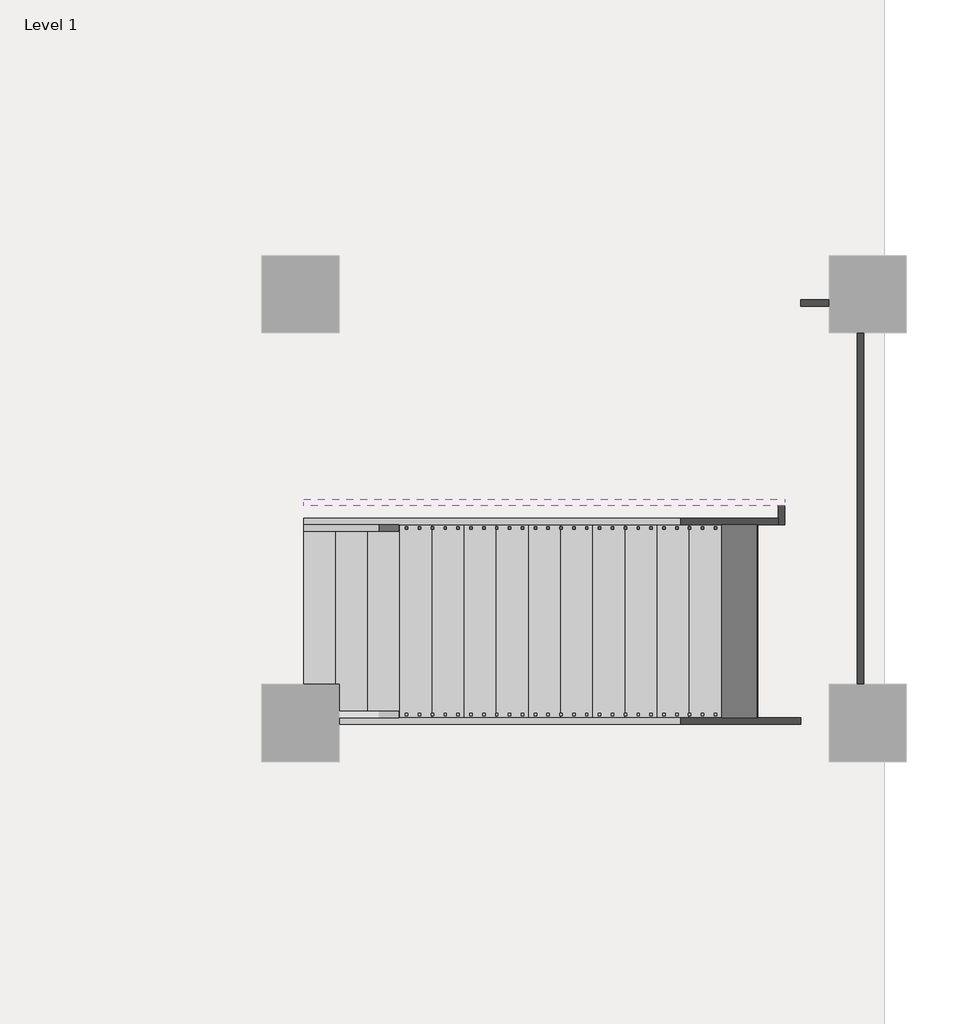
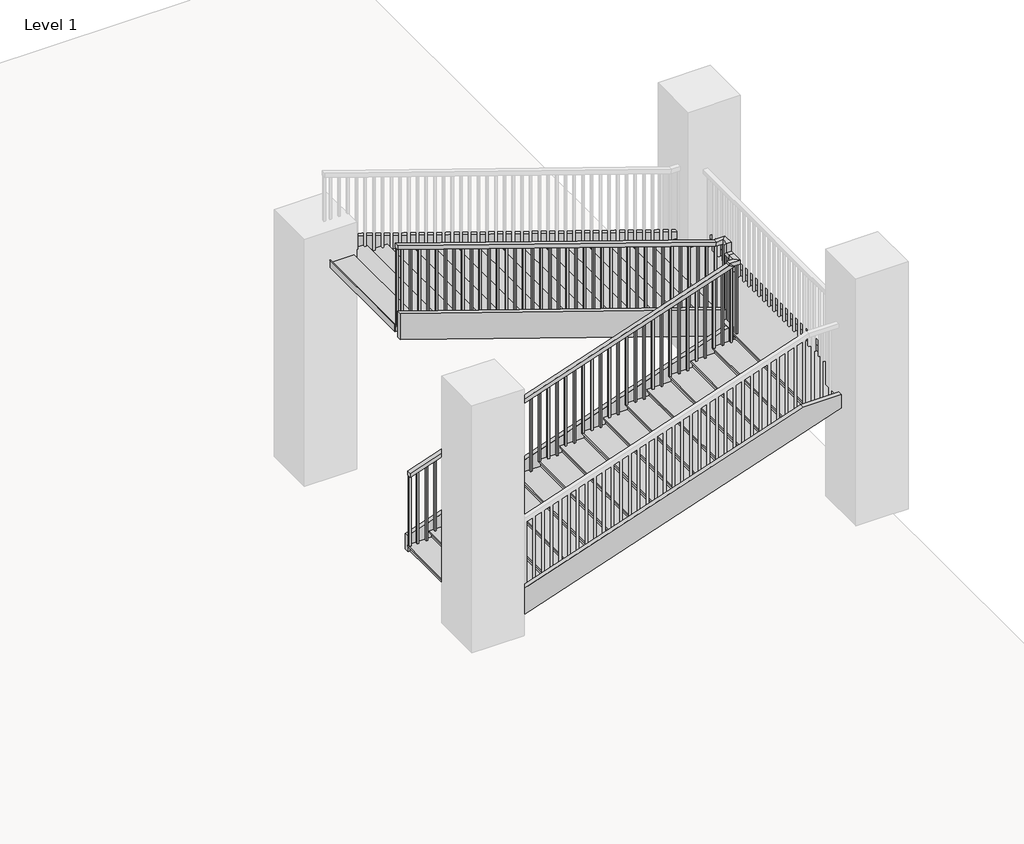
# One storey, part 2 of 2: 6 members, 1 railing, 1 stair flight.
"""IFC4 building model written with IfcOpenShell, lengths in millimetres."""

from ifc_helpers import new_model, si_unit, frame, origin, place, context, project, spatial, polyline, outline, extrude, faceted_brep, transform, mapped, element, save
from components import stair_flight_62363484

model = new_model("IFC4")

# Units and contexts
model_context = context("Model", 3, world=origin())
ifc_project = project(units=[si_unit("LENGTHUNIT", "METRE", prefix="MILLI")], contexts=[model_context])

# Site, building, storey
site = spatial("IfcSite", under=ifc_project)
building = spatial("IfcBuilding", under=site)
storey = spatial("IfcBuildingStorey", under=building, Name="Level 1", Elevation=0.0)

# Members
placement = place(None, origin())
element("IfcMember", 1, ObjectType="Stringer - 2\" Width", at=placement, inside=storey, context=model_context, shape_type="SweptSolid", body=[
    extrude(outline(polyline([(193.7751932, 1449.3932247), (0.0, 1449.3932247), (0.0, 1827.5890963), (1140.094539, 5195.8669505), (1447.8, 5195.8669505), (1447.8, 5154.2649181), (193.7751932, 1449.3932247)])), frame((0.0, -541.2659014, 0.0), z_axis=(0.0, 1.0, 0.0), x_axis=(0.0, 0.0, 1.0)), (0.0, 0.0, 1.0), 50.8),
])
element("IfcMember", 2, ObjectType="Stringer - 2\" Width", at=placement, inside=storey, context=model_context, shape_type="SweptSolid", body=[
    extrude(outline(polyline([(5246.6669505, -541.2659014), (5195.8669505, -541.2659014), (5195.8669505, -388.7910016), (5246.6669505, -388.7910016), (5246.6669505, -541.2659014)])), frame((0.0, 0.0, 1143.0), z_axis=(0.0, 0.0, 1.0), x_axis=(1.0, 0.0, 0.0)), (0.0, 0.0, 1.0), 304.8),
])
element("IfcMember", 3, ObjectType="Stringer - 2\" Width", at=placement, inside=storey, context=model_context, shape_type="SweptSolid", body=[
    extrude(outline(polyline([(1243.0143208, 5246.6669505), (1564.8012358, 5246.6669505), (2850.1022784, 1449.3932247), (2528.3153634, 1449.3932247), (1243.0143208, 5246.6669505)])), frame((0.0, -388.7910016, 0.0), z_axis=(0.0, 1.0, 0.0), x_axis=(0.0, 0.0, 1.0)), (0.0, 0.0, 1.0), 50.8),
])
element("IfcMember", 4, ObjectType="Stringer - 2\" Width", at=placement, inside=storey, context=model_context, shape_type="SweptSolid", body=[
    extrude(outline(polyline([(193.7751932, 1449.3932247), (0.0, 1449.3932247), (0.0, 1827.5890963), (1352.1142723, 5822.2548051), (1447.8, 5822.2548051), (1447.8, 5154.2649181), (193.7751932, 1449.3932247)])), frame((0.0, -2116.0659014, 0.0), z_axis=(0.0, 1.0, 0.0), x_axis=(0.0, 0.0, 1.0)), (0.0, 0.0, 1.0), 50.8),
])
element("IfcMember", 5, ObjectType="Stringer - 2\" Width", at=placement, inside=storey, context=model_context, shape_type="SweptSolid", body=[
    extrude(outline(polyline([(5873.0548051, -2116.0659014), (5822.2548051, -2116.0659014), (5822.2548051, 1185.9340986), (5873.0548051, 1185.9340986), (5873.0548051, -2116.0659014)])), frame((0.0, 0.0, 1143.0), z_axis=(0.0, 0.0, 1.0), x_axis=(1.0, 0.0, 0.0)), (0.0, 0.0, 1.0), 304.8),
])
element("IfcMember", 6, ObjectType="Stringer - 2\" Width", at=placement, inside=storey, context=model_context, shape_type="SweptSolid", body=[
    extrude(outline(polyline([(1143.0, 5873.0548051), (1352.7815025, 5873.0548051), (2850.1022784, 1449.3932247), (2528.3153634, 1449.3932247), (1143.0, 5542.1477288), (1143.0, 5873.0548051)])), frame((0.0, 1185.9340986, 0.0), z_axis=(0.0, 1.0, 0.0), x_axis=(0.0, 0.0, 1.0)), (0.0, 0.0, 1.0), 50.8),
])

# Railing
element("IfcRailing", 7, ObjectType="Handrail - Rectangular", at=placement, inside=storey, context=model_context, shape_type="SolidModel", body=[
    faceted_brep([(1449.3932247, -541.2659014, 1000.125), (1449.3932247, -541.2659014, 946.4913852), (1449.3932247, -592.0659014, 946.4913852), (1449.3932247, -592.0659014, 1000.125), (5170.4669505, -541.2659014, 2260.1963098), (5221.2669505, -541.2659014, 2223.7651551), (5221.2669505, -592.0659014, 2223.7651551), (5170.4669505, -592.0659014, 2260.1963098), (5170.4669505, -541.2659014, 2286.0), (5221.2669505, -541.2659014, 2235.2), (5221.2669505, -592.0659014, 2235.2), (5170.4669505, -592.0659014, 2286.0), (5246.6669505, -541.2659014, 2286.0), (5246.6669505, -541.2659014, 2235.2), (5297.4669505, -592.0659014, 2235.2), (5297.4669505, -592.0659014, 2286.0), (5246.6669505, -465.0659014, 2286.0), (5246.6669505, -465.0659014, 2235.2), (5297.4669505, -465.0659014, 2235.2), (5297.4669505, -465.0659014, 2286.0), (5246.6669505, -414.1910016, 2286.0), (5246.6669505, -363.3910016, 2235.2), (5297.4669505, -363.3910016, 2235.2), (5297.4669505, -414.1910016, 2286.0), (5246.6669505, -414.1910016, 2397.5286902), (5246.6669505, -363.3910016, 2346.7286902), (5297.4669505, -363.3910016, 2346.7286902), (5297.4669505, -414.1910016, 2397.5286902), (5246.6669505, -337.9910016, 2397.5286902), (5246.6669505, -337.9910016, 2346.7286902), (5297.4669505, -287.1910016, 2346.7286902), (5297.4669505, -287.1910016, 2397.5286902), (5170.4669505, -337.9910016, 2397.5286902), (5162.099099, -337.9910016, 2346.7286902), (5162.099099, -287.1910016, 2346.7286902), (5170.4669505, -287.1910016, 2397.5286902), (1449.3932247, -337.9910016, 3657.6), (1449.3932247, -287.1910016, 3657.6), (1449.3932247, -287.1910016, 3603.9663852), (1449.3932247, -337.9910016, 3603.9663852)], [[[0, 1, 2, 3]], [[1, 0, 4, 5]], [[2, 1, 5, 6]], [[3, 2, 6, 7]], [[0, 3, 7, 4]], [[5, 4, 8, 9]], [[6, 5, 9, 10]], [[7, 6, 10, 11]], [[4, 7, 11, 8]], [[9, 8, 12, 13]], [[10, 9, 13, 14]], [[11, 10, 14, 15]], [[8, 11, 15, 12]], [[13, 12, 16, 17]], [[14, 13, 17, 18]], [[15, 14, 18, 19]], [[12, 15, 19, 16]], [[17, 16, 20, 21]], [[18, 17, 21, 22]], [[19, 18, 22, 23]], [[16, 19, 23, 20]], [[21, 20, 24, 25]], [[22, 21, 25, 26]], [[23, 22, 26, 27]], [[20, 23, 27, 24]], [[25, 24, 28, 29]], [[26, 25, 29, 30]], [[27, 26, 30, 31]], [[24, 27, 31, 28]], [[29, 28, 32, 33]], [[30, 29, 33, 34]], [[31, 30, 34, 35]], [[28, 31, 35, 32]], [[36, 37, 38, 39]], [[33, 32, 36, 39]], [[34, 33, 39, 38]], [[35, 34, 38, 37]], [[32, 35, 37, 36]]]),
    extrude(outline(polyline([(3585.6976686, 1503.3419505), (2657.475, 1503.3419505), (2657.475, 1522.3919505), (3579.246746, 1522.3919505), (3585.6976686, 1503.3419505)])), frame((0.0, -322.1160016, 0.0), z_axis=(0.0, 1.0, 0.0), x_axis=(0.0, 0.0, 1.0)), (0.0, 0.0, 1.0), 19.05),
    extrude(outline(polyline([(3551.2927482, 1604.9419505), (2657.475, 1604.9419505), (2657.475, 1623.9919505), (3544.8418257, 1623.9919505), (3551.2927482, 1604.9419505)])), frame((0.0, -322.1160016, 0.0), z_axis=(0.0, 1.0, 0.0), x_axis=(0.0, 0.0, 1.0)), (0.0, 0.0, 1.0), 19.05),
    extrude(outline(polyline([(3516.8878279, 1706.5419505), (2571.75, 1706.5419505), (2571.75, 1725.5919505), (3510.4369054, 1725.5919505), (3516.8878279, 1706.5419505)])), frame((0.0, -322.1160016, 0.0), z_axis=(0.0, 1.0, 0.0), x_axis=(0.0, 0.0, 1.0)), (0.0, 0.0, 1.0), 19.05),
    extrude(outline(polyline([(3482.4829076, 1808.1419505), (2571.75, 1808.1419505), (2571.75, 1827.1919505), (3476.031985, 1827.1919505), (3482.4829076, 1808.1419505)])), frame((0.0, -322.1160016, 0.0), z_axis=(0.0, 1.0, 0.0), x_axis=(0.0, 0.0, 1.0)), (0.0, 0.0, 1.0), 19.05),
    extrude(outline(polyline([(3448.0779873, 1909.7419505), (2571.75, 1909.7419505), (2571.75, 1928.7919505), (3441.6270647, 1928.7919505), (3448.0779873, 1909.7419505)])), frame((0.0, -322.1160016, 0.0), z_axis=(0.0, 1.0, 0.0), x_axis=(0.0, 0.0, 1.0)), (0.0, 0.0, 1.0), 19.05),
    extrude(outline(polyline([(3413.6730669, 2011.3419505), (2486.025, 2011.3419505), (2486.025, 2030.3919505), (3407.2221444, 2030.3919505), (3413.6730669, 2011.3419505)])), frame((0.0, -322.1160016, 0.0), z_axis=(0.0, 1.0, 0.0), x_axis=(0.0, 0.0, 1.0)), (0.0, 0.0, 1.0), 19.05),
    extrude(outline(polyline([(3379.2681466, 2112.9419505), (2486.025, 2112.9419505), (2486.025, 2131.9919505), (3372.817224, 2131.9919505), (3379.2681466, 2112.9419505)])), frame((0.0, -322.1160016, 0.0), z_axis=(0.0, 1.0, 0.0), x_axis=(0.0, 0.0, 1.0)), (0.0, 0.0, 1.0), 19.05),
    extrude(outline(polyline([(3344.8632263, 2214.5419505), (2400.3, 2214.5419505), (2400.3, 2233.5919505), (3338.4123037, 2233.5919505), (3344.8632263, 2214.5419505)])), frame((0.0, -322.1160016, 0.0), z_axis=(0.0, 1.0, 0.0), x_axis=(0.0, 0.0, 1.0)), (0.0, 0.0, 1.0), 19.05),
    extrude(outline(polyline([(3310.4583059, 2316.1419505), (2400.3, 2316.1419505), (2400.3, 2335.1919505), (3304.0073834, 2335.1919505), (3310.4583059, 2316.1419505)])), frame((0.0, -322.1160016, 0.0), z_axis=(0.0, 1.0, 0.0), x_axis=(0.0, 0.0, 1.0)), (0.0, 0.0, 1.0), 19.05),
    extrude(outline(polyline([(3276.0533856, 2417.7419505), (2400.3, 2417.7419505), (2400.3, 2436.7919505), (3269.6024631, 2436.7919505), (3276.0533856, 2417.7419505)])), frame((0.0, -322.1160016, 0.0), z_axis=(0.0, 1.0, 0.0), x_axis=(0.0, 0.0, 1.0)), (0.0, 0.0, 1.0), 19.05),
    extrude(outline(polyline([(3241.6484653, 2519.3419505), (2314.575, 2519.3419505), (2314.575, 2538.3919505), (3235.1975427, 2538.3919505), (3241.6484653, 2519.3419505)])), frame((0.0, -322.1160016, 0.0), z_axis=(0.0, 1.0, 0.0), x_axis=(0.0, 0.0, 1.0)), (0.0, 0.0, 1.0), 19.05),
    extrude(outline(polyline([(3207.243545, 2620.9419505), (2314.575, 2620.9419505), (2314.575, 2639.9919505), (3200.7926224, 2639.9919505), (3207.243545, 2620.9419505)])), frame((0.0, -322.1160016, 0.0), z_axis=(0.0, 1.0, 0.0), x_axis=(0.0, 0.0, 1.0)), (0.0, 0.0, 1.0), 19.05),
    extrude(outline(polyline([(3172.8386246, 2722.5419505), (2228.85, 2722.5419505), (2228.85, 2741.5919505), (3166.3877021, 2741.5919505), (3172.8386246, 2722.5419505)])), frame((0.0, -322.1160016, 0.0), z_axis=(0.0, 1.0, 0.0), x_axis=(0.0, 0.0, 1.0)), (0.0, 0.0, 1.0), 19.05),
    extrude(outline(polyline([(3138.4337043, 2824.1419505), (2228.85, 2824.1419505), (2228.85, 2843.1919505), (3131.9827817, 2843.1919505), (3138.4337043, 2824.1419505)])), frame((0.0, -322.1160016, 0.0), z_axis=(0.0, 1.0, 0.0), x_axis=(0.0, 0.0, 1.0)), (0.0, 0.0, 1.0), 19.05),
    extrude(outline(polyline([(3104.028784, 2925.7419505), (2228.85, 2925.7419505), (2228.85, 2944.7919505), (3097.5778614, 2944.7919505), (3104.028784, 2925.7419505)])), frame((0.0, -322.1160016, 0.0), z_axis=(0.0, 1.0, 0.0), x_axis=(0.0, 0.0, 1.0)), (0.0, 0.0, 1.0), 19.05),
    extrude(outline(polyline([(3069.6238636, 3027.3419505), (2143.125, 3027.3419505), (2143.125, 3046.3919505), (3063.1729411, 3046.3919505), (3069.6238636, 3027.3419505)])), frame((0.0, -322.1160016, 0.0), z_axis=(0.0, 1.0, 0.0), x_axis=(0.0, 0.0, 1.0)), (0.0, 0.0, 1.0), 19.05),
    extrude(outline(polyline([(3035.2189433, 3128.9419505), (2143.125, 3128.9419505), (2143.125, 3147.9919505), (3028.7680208, 3147.9919505), (3035.2189433, 3128.9419505)])), frame((0.0, -322.1160016, 0.0), z_axis=(0.0, 1.0, 0.0), x_axis=(0.0, 0.0, 1.0)), (0.0, 0.0, 1.0), 19.05),
    extrude(outline(polyline([(3000.814023, 3230.5419505), (2057.4, 3230.5419505), (2057.4, 3249.5919505), (2994.3631004, 3249.5919505), (3000.814023, 3230.5419505)])), frame((0.0, -322.1160016, 0.0), z_axis=(0.0, 1.0, 0.0), x_axis=(0.0, 0.0, 1.0)), (0.0, 0.0, 1.0), 19.05),
    extrude(outline(polyline([(2966.4091027, 3332.1419505), (2057.4, 3332.1419505), (2057.4, 3351.1919505), (2959.9581801, 3351.1919505), (2966.4091027, 3332.1419505)])), frame((0.0, -322.1160016, 0.0), z_axis=(0.0, 1.0, 0.0), x_axis=(0.0, 0.0, 1.0)), (0.0, 0.0, 1.0), 19.05),
    extrude(outline(polyline([(2932.0041823, 3433.7419505), (2057.4, 3433.7419505), (2057.4, 3452.7919505), (2925.5532598, 3452.7919505), (2932.0041823, 3433.7419505)])), frame((0.0, -322.1160016, 0.0), z_axis=(0.0, 1.0, 0.0), x_axis=(0.0, 0.0, 1.0)), (0.0, 0.0, 1.0), 19.05),
    extrude(outline(polyline([(2897.599262, 3535.3419505), (1971.675, 3535.3419505), (1971.675, 3554.3919505), (2891.1483394, 3554.3919505), (2897.599262, 3535.3419505)])), frame((0.0, -322.1160016, 0.0), z_axis=(0.0, 1.0, 0.0), x_axis=(0.0, 0.0, 1.0)), (0.0, 0.0, 1.0), 19.05),
    extrude(outline(polyline([(2863.1943417, 3636.9419505), (1971.675, 3636.9419505), (1971.675, 3655.9919505), (2856.7434191, 3655.9919505), (2863.1943417, 3636.9419505)])), frame((0.0, -322.1160016, 0.0), z_axis=(0.0, 1.0, 0.0), x_axis=(0.0, 0.0, 1.0)), (0.0, 0.0, 1.0), 19.05),
    extrude(outline(polyline([(2828.7894213, 3738.5419505), (1885.95, 3738.5419505), (1885.95, 3757.5919505), (2822.3384988, 3757.5919505), (2828.7894213, 3738.5419505)])), frame((0.0, -322.1160016, 0.0), z_axis=(0.0, 1.0, 0.0), x_axis=(0.0, 0.0, 1.0)), (0.0, 0.0, 1.0), 19.05),
    extrude(outline(polyline([(2794.384501, 3840.1419505), (1885.95, 3840.1419505), (1885.95, 3859.1919505), (2787.9335784, 3859.1919505), (2794.384501, 3840.1419505)])), frame((0.0, -322.1160016, 0.0), z_axis=(0.0, 1.0, 0.0), x_axis=(0.0, 0.0, 1.0)), (0.0, 0.0, 1.0), 19.05),
    extrude(outline(polyline([(2759.9795807, 3941.7419505), (1885.95, 3941.7419505), (1885.95, 3960.7919505), (2753.5286581, 3960.7919505), (2759.9795807, 3941.7419505)])), frame((0.0, -322.1160016, 0.0), z_axis=(0.0, 1.0, 0.0), x_axis=(0.0, 0.0, 1.0)), (0.0, 0.0, 1.0), 19.05),
    extrude(outline(polyline([(2725.5746604, 4043.3419505), (1800.225, 4043.3419505), (1800.225, 4062.3919505), (2719.1237378, 4062.3919505), (2725.5746604, 4043.3419505)])), frame((0.0, -322.1160016, 0.0), z_axis=(0.0, 1.0, 0.0), x_axis=(0.0, 0.0, 1.0)), (0.0, 0.0, 1.0), 19.05),
    extrude(outline(polyline([(2691.16974, 4144.9419505), (1800.225, 4144.9419505), (1800.225, 4163.9919505), (2684.7188175, 4163.9919505), (2691.16974, 4144.9419505)])), frame((0.0, -322.1160016, 0.0), z_axis=(0.0, 1.0, 0.0), x_axis=(0.0, 0.0, 1.0)), (0.0, 0.0, 1.0), 19.05),
    extrude(outline(polyline([(2656.7648197, 4246.5419505), (1714.5, 4246.5419505), (1714.5, 4265.5919505), (2650.3138971, 4265.5919505), (2656.7648197, 4246.5419505)])), frame((0.0, -322.1160016, 0.0), z_axis=(0.0, 1.0, 0.0), x_axis=(0.0, 0.0, 1.0)), (0.0, 0.0, 1.0), 19.05),
    extrude(outline(polyline([(2622.3598994, 4348.1419505), (1714.5, 4348.1419505), (1714.5, 4367.1919505), (2615.9089768, 4367.1919505), (2622.3598994, 4348.1419505)])), frame((0.0, -322.1160016, 0.0), z_axis=(0.0, 1.0, 0.0), x_axis=(0.0, 0.0, 1.0)), (0.0, 0.0, 1.0), 19.05),
    extrude(outline(polyline([(2587.954979, 4449.7419505), (1714.5, 4449.7419505), (1714.5, 4468.7919505), (2581.5040565, 4468.7919505), (2587.954979, 4449.7419505)])), frame((0.0, -322.1160016, 0.0), z_axis=(0.0, 1.0, 0.0), x_axis=(0.0, 0.0, 1.0)), (0.0, 0.0, 1.0), 19.05),
    extrude(outline(polyline([(2553.5500587, 4551.3419505), (1628.775, 4551.3419505), (1628.775, 4570.3919505), (2547.0991361, 4570.3919505), (2553.5500587, 4551.3419505)])), frame((0.0, -322.1160016, 0.0), z_axis=(0.0, 1.0, 0.0), x_axis=(0.0, 0.0, 1.0)), (0.0, 0.0, 1.0), 19.05),
    extrude(outline(polyline([(2519.1451384, 4652.9419505), (1628.775, 4652.9419505), (1628.775, 4671.9919505), (2512.6942158, 4671.9919505), (2519.1451384, 4652.9419505)])), frame((0.0, -322.1160016, 0.0), z_axis=(0.0, 1.0, 0.0), x_axis=(0.0, 0.0, 1.0)), (0.0, 0.0, 1.0), 19.05),
    extrude(outline(polyline([(2484.7402181, 4754.5419505), (1543.05, 4754.5419505), (1543.05, 4773.5919505), (2478.2892955, 4773.5919505), (2484.7402181, 4754.5419505)])), frame((0.0, -322.1160016, 0.0), z_axis=(0.0, 1.0, 0.0), x_axis=(0.0, 0.0, 1.0)), (0.0, 0.0, 1.0), 19.05),
    extrude(outline(polyline([(2450.3352977, 4856.1419505), (1543.05, 4856.1419505), (1543.05, 4875.1919505), (2443.8843752, 4875.1919505), (2450.3352977, 4856.1419505)])), frame((0.0, -322.1160016, 0.0), z_axis=(0.0, 1.0, 0.0), x_axis=(0.0, 0.0, 1.0)), (0.0, 0.0, 1.0), 19.05),
    extrude(outline(polyline([(2415.9303774, 4957.7419505), (1543.05, 4957.7419505), (1543.05, 4976.7919505), (2409.4794548, 4976.7919505), (2415.9303774, 4957.7419505)])), frame((0.0, -322.1160016, 0.0), z_axis=(0.0, 1.0, 0.0), x_axis=(0.0, 0.0, 1.0)), (0.0, 0.0, 1.0), 19.05),
    extrude(outline(polyline([(2381.5254571, 5059.3419505), (1457.325, 5059.3419505), (1457.325, 5078.3919505), (2375.0745345, 5078.3919505), (2381.5254571, 5059.3419505)])), frame((0.0, -322.1160016, 0.0), z_axis=(0.0, 1.0, 0.0), x_axis=(0.0, 0.0, 1.0)), (0.0, 0.0, 1.0), 19.05),
    extrude(outline(polyline([(2347.1205367, 5160.9419505), (1457.325, 5160.9419505), (1457.325, 5179.9919505), (2340.6696142, 5179.9919505), (2347.1205367, 5160.9419505)])), frame((0.0, -322.1160016, 0.0), z_axis=(0.0, 1.0, 0.0), x_axis=(0.0, 0.0, 1.0)), (0.0, 0.0, 1.0), 19.05),
    extrude(outline(polyline([(5262.5419505, -372.9909014), (5262.5419505, -353.9409014), (5281.5919505, -353.9409014), (5281.5919505, -372.9909014), (5262.5419505, -372.9909014)])), frame((0.0, 0.0, 1371.6), z_axis=(0.0, 0.0, 1.0), x_axis=(1.0, 0.0, 0.0)), (0.0, 0.0, 1.0), 975.1286902),
    extrude(outline(polyline([(5262.5419505, -474.5909014), (5262.5419505, -455.5409014), (5281.5919505, -455.5409014), (5281.5919505, -474.5909014), (5262.5419505, -474.5909014)])), frame((0.0, 0.0, 1371.6), z_axis=(0.0, 0.0, 1.0), x_axis=(1.0, 0.0, 0.0)), (0.0, 0.0, 1.0), 863.6),
    extrude(outline(polyline([(5199.0682247, -557.1409014), (5218.1182247, -557.1409014), (5218.1182247, -576.1909014), (5199.0682247, -576.1909014), (5199.0682247, -557.1409014)])), frame((0.0, 0.0, 1285.875), z_axis=(0.0, 0.0, 1.0), x_axis=(1.0, 0.0, 0.0)), (0.0, 0.0, 1.0), 949.325),
    extrude(outline(polyline([(2181.8430558, 5097.4682247), (1285.875, 5097.4682247), (1285.875, 5116.5182247), (2188.2939783, 5116.5182247), (2181.8430558, 5097.4682247)])), frame((0.0, -576.1909014, 0.0), z_axis=(0.0, 1.0, 0.0), x_axis=(0.0, 0.0, 1.0)), (0.0, 0.0, 1.0), 19.05),
    extrude(outline(polyline([(2147.4381354, 4995.8682247), (1285.875, 4995.8682247), (1285.875, 5014.9182247), (2153.889058, 5014.9182247), (2147.4381354, 4995.8682247)])), frame((0.0, -576.1909014, 0.0), z_axis=(0.0, 1.0, 0.0), x_axis=(0.0, 0.0, 1.0)), (0.0, 0.0, 1.0), 19.05),
    extrude(outline(polyline([(2113.0332151, 4894.2682247), (1200.15, 4894.2682247), (1200.15, 4913.3182247), (2119.4841377, 4913.3182247), (2113.0332151, 4894.2682247)])), frame((0.0, -576.1909014, 0.0), z_axis=(0.0, 1.0, 0.0), x_axis=(0.0, 0.0, 1.0)), (0.0, 0.0, 1.0), 19.05),
    extrude(outline(polyline([(2078.6282948, 4792.6682247), (1200.15, 4792.6682247), (1200.15, 4811.7182247), (2085.0792173, 4811.7182247), (2078.6282948, 4792.6682247)])), frame((0.0, -576.1909014, 0.0), z_axis=(0.0, 1.0, 0.0), x_axis=(0.0, 0.0, 1.0)), (0.0, 0.0, 1.0), 19.05),
    extrude(outline(polyline([(2044.2233745, 4691.0682247), (1114.425, 4691.0682247), (1114.425, 4710.1182247), (2050.674297, 4710.1182247), (2044.2233745, 4691.0682247)])), frame((0.0, -576.1909014, 0.0), z_axis=(0.0, 1.0, 0.0), x_axis=(0.0, 0.0, 1.0)), (0.0, 0.0, 1.0), 19.05),
    extrude(outline(polyline([(2009.8184541, 4589.4682247), (1114.425, 4589.4682247), (1114.425, 4608.5182247), (2016.2693767, 4608.5182247), (2009.8184541, 4589.4682247)])), frame((0.0, -576.1909014, 0.0), z_axis=(0.0, 1.0, 0.0), x_axis=(0.0, 0.0, 1.0)), (0.0, 0.0, 1.0), 19.05),
    extrude(outline(polyline([(1975.4135338, 4487.8682247), (1114.425, 4487.8682247), (1114.425, 4506.9182247), (1981.8644564, 4506.9182247), (1975.4135338, 4487.8682247)])), frame((0.0, -576.1909014, 0.0), z_axis=(0.0, 1.0, 0.0), x_axis=(0.0, 0.0, 1.0)), (0.0, 0.0, 1.0), 19.05),
    extrude(outline(polyline([(1941.0086135, 4386.2682247), (1028.7, 4386.2682247), (1028.7, 4405.3182247), (1947.459536, 4405.3182247), (1941.0086135, 4386.2682247)])), frame((0.0, -576.1909014, 0.0), z_axis=(0.0, 1.0, 0.0), x_axis=(0.0, 0.0, 1.0)), (0.0, 0.0, 1.0), 19.05),
    extrude(outline(polyline([(1906.6036931, 4284.6682247), (1028.7, 4284.6682247), (1028.7, 4303.7182247), (1913.0546157, 4303.7182247), (1906.6036931, 4284.6682247)])), frame((0.0, -576.1909014, 0.0), z_axis=(0.0, 1.0, 0.0), x_axis=(0.0, 0.0, 1.0)), (0.0, 0.0, 1.0), 19.05),
    extrude(outline(polyline([(1872.1987728, 4183.0682247), (942.975, 4183.0682247), (942.975, 4202.1182247), (1878.6496954, 4202.1182247), (1872.1987728, 4183.0682247)])), frame((0.0, -576.1909014, 0.0), z_axis=(0.0, 1.0, 0.0), x_axis=(0.0, 0.0, 1.0)), (0.0, 0.0, 1.0), 19.05),
    extrude(outline(polyline([(1837.7938525, 4081.4682247), (942.975, 4081.4682247), (942.975, 4100.5182247), (1844.244775, 4100.5182247), (1837.7938525, 4081.4682247)])), frame((0.0, -576.1909014, 0.0), z_axis=(0.0, 1.0, 0.0), x_axis=(0.0, 0.0, 1.0)), (0.0, 0.0, 1.0), 19.05),
    extrude(outline(polyline([(1803.3889321, 3979.8682247), (942.975, 3979.8682247), (942.975, 3998.9182247), (1809.8398547, 3998.9182247), (1803.3889321, 3979.8682247)])), frame((0.0, -576.1909014, 0.0), z_axis=(0.0, 1.0, 0.0), x_axis=(0.0, 0.0, 1.0)), (0.0, 0.0, 1.0), 19.05),
    extrude(outline(polyline([(1768.9840118, 3878.2682247), (857.25, 3878.2682247), (857.25, 3897.3182247), (1775.4349344, 3897.3182247), (1768.9840118, 3878.2682247)])), frame((0.0, -576.1909014, 0.0), z_axis=(0.0, 1.0, 0.0), x_axis=(0.0, 0.0, 1.0)), (0.0, 0.0, 1.0), 19.05),
    extrude(outline(polyline([(1734.5790915, 3776.6682247), (857.25, 3776.6682247), (857.25, 3795.7182247), (1741.0300141, 3795.7182247), (1734.5790915, 3776.6682247)])), frame((0.0, -576.1909014, 0.0), z_axis=(0.0, 1.0, 0.0), x_axis=(0.0, 0.0, 1.0)), (0.0, 0.0, 1.0), 19.05),
    extrude(outline(polyline([(1700.1741712, 3675.0682247), (771.525, 3675.0682247), (771.525, 3694.1182247), (1706.6250937, 3694.1182247), (1700.1741712, 3675.0682247)])), frame((0.0, -576.1909014, 0.0), z_axis=(0.0, 1.0, 0.0), x_axis=(0.0, 0.0, 1.0)), (0.0, 0.0, 1.0), 19.05),
    extrude(outline(polyline([(1665.7692508, 3573.4682247), (771.525, 3573.4682247), (771.525, 3592.5182247), (1672.2201734, 3592.5182247), (1665.7692508, 3573.4682247)])), frame((0.0, -576.1909014, 0.0), z_axis=(0.0, 1.0, 0.0), x_axis=(0.0, 0.0, 1.0)), (0.0, 0.0, 1.0), 19.05),
    extrude(outline(polyline([(1631.3643305, 3471.8682247), (771.525, 3471.8682247), (771.525, 3490.9182247), (1637.8152531, 3490.9182247), (1631.3643305, 3471.8682247)])), frame((0.0, -576.1909014, 0.0), z_axis=(0.0, 1.0, 0.0), x_axis=(0.0, 0.0, 1.0)), (0.0, 0.0, 1.0), 19.05),
    extrude(outline(polyline([(1596.9594102, 3370.2682247), (685.8, 3370.2682247), (685.8, 3389.3182247), (1603.4103327, 3389.3182247), (1596.9594102, 3370.2682247)])), frame((0.0, -576.1909014, 0.0), z_axis=(0.0, 1.0, 0.0), x_axis=(0.0, 0.0, 1.0)), (0.0, 0.0, 1.0), 19.05),
    extrude(outline(polyline([(1562.5544898, 3268.6682247), (685.8, 3268.6682247), (685.8, 3287.7182247), (1569.0054124, 3287.7182247), (1562.5544898, 3268.6682247)])), frame((0.0, -576.1909014, 0.0), z_axis=(0.0, 1.0, 0.0), x_axis=(0.0, 0.0, 1.0)), (0.0, 0.0, 1.0), 19.05),
    extrude(outline(polyline([(1528.1495695, 3167.0682247), (600.075, 3167.0682247), (600.075, 3186.1182247), (1534.6004921, 3186.1182247), (1528.1495695, 3167.0682247)])), frame((0.0, -576.1909014, 0.0), z_axis=(0.0, 1.0, 0.0), x_axis=(0.0, 0.0, 1.0)), (0.0, 0.0, 1.0), 19.05),
    extrude(outline(polyline([(1493.7446492, 3065.4682247), (600.075, 3065.4682247), (600.075, 3084.5182247), (1500.1955718, 3084.5182247), (1493.7446492, 3065.4682247)])), frame((0.0, -576.1909014, 0.0), z_axis=(0.0, 1.0, 0.0), x_axis=(0.0, 0.0, 1.0)), (0.0, 0.0, 1.0), 19.05),
    extrude(outline(polyline([(1459.3397289, 2963.8682247), (600.075, 2963.8682247), (600.075, 2982.9182247), (1465.7906514, 2982.9182247), (1459.3397289, 2963.8682247)])), frame((0.0, -576.1909014, 0.0), z_axis=(0.0, 1.0, 0.0), x_axis=(0.0, 0.0, 1.0)), (0.0, 0.0, 1.0), 19.05),
    extrude(outline(polyline([(1424.9348085, 2862.2682247), (514.35, 2862.2682247), (514.35, 2881.3182247), (1431.3857311, 2881.3182247), (1424.9348085, 2862.2682247)])), frame((0.0, -576.1909014, 0.0), z_axis=(0.0, 1.0, 0.0), x_axis=(0.0, 0.0, 1.0)), (0.0, 0.0, 1.0), 19.05),
    extrude(outline(polyline([(1390.5298882, 2760.6682247), (514.35, 2760.6682247), (514.35, 2779.7182247), (1396.9808108, 2779.7182247), (1390.5298882, 2760.6682247)])), frame((0.0, -576.1909014, 0.0), z_axis=(0.0, 1.0, 0.0), x_axis=(0.0, 0.0, 1.0)), (0.0, 0.0, 1.0), 19.05),
    extrude(outline(polyline([(1356.1249679, 2659.0682247), (428.625, 2659.0682247), (428.625, 2678.1182247), (1362.5758904, 2678.1182247), (1356.1249679, 2659.0682247)])), frame((0.0, -576.1909014, 0.0), z_axis=(0.0, 1.0, 0.0), x_axis=(0.0, 0.0, 1.0)), (0.0, 0.0, 1.0), 19.05),
    extrude(outline(polyline([(1321.7200475, 2557.4682247), (428.625, 2557.4682247), (428.625, 2576.5182247), (1328.1709701, 2576.5182247), (1321.7200475, 2557.4682247)])), frame((0.0, -576.1909014, 0.0), z_axis=(0.0, 1.0, 0.0), x_axis=(0.0, 0.0, 1.0)), (0.0, 0.0, 1.0), 19.05),
    extrude(outline(polyline([(1287.3151272, 2455.8682247), (428.625, 2455.8682247), (428.625, 2474.9182247), (1293.7660498, 2474.9182247), (1287.3151272, 2455.8682247)])), frame((0.0, -576.1909014, 0.0), z_axis=(0.0, 1.0, 0.0), x_axis=(0.0, 0.0, 1.0)), (0.0, 0.0, 1.0), 19.05),
    extrude(outline(polyline([(1252.9102069, 2354.2682247), (342.9, 2354.2682247), (342.9, 2373.3182247), (1259.3611294, 2373.3182247), (1252.9102069, 2354.2682247)])), frame((0.0, -576.1909014, 0.0), z_axis=(0.0, 1.0, 0.0), x_axis=(0.0, 0.0, 1.0)), (0.0, 0.0, 1.0), 19.05),
    extrude(outline(polyline([(1218.5052866, 2252.6682247), (342.9, 2252.6682247), (342.9, 2271.7182247), (1224.9562091, 2271.7182247), (1218.5052866, 2252.6682247)])), frame((0.0, -576.1909014, 0.0), z_axis=(0.0, 1.0, 0.0), x_axis=(0.0, 0.0, 1.0)), (0.0, 0.0, 1.0), 19.05),
    extrude(outline(polyline([(1184.1003662, 2151.0682247), (257.175, 2151.0682247), (257.175, 2170.1182247), (1190.5512888, 2170.1182247), (1184.1003662, 2151.0682247)])), frame((0.0, -576.1909014, 0.0), z_axis=(0.0, 1.0, 0.0), x_axis=(0.0, 0.0, 1.0)), (0.0, 0.0, 1.0), 19.05),
    extrude(outline(polyline([(1149.6954459, 2049.4682247), (257.175, 2049.4682247), (257.175, 2068.5182247), (1156.1463685, 2068.5182247), (1149.6954459, 2049.4682247)])), frame((0.0, -576.1909014, 0.0), z_axis=(0.0, 1.0, 0.0), x_axis=(0.0, 0.0, 1.0)), (0.0, 0.0, 1.0), 19.05),
    extrude(outline(polyline([(1115.2905256, 1947.8682247), (257.175, 1947.8682247), (257.175, 1966.9182247), (1121.7414481, 1966.9182247), (1115.2905256, 1947.8682247)])), frame((0.0, -576.1909014, 0.0), z_axis=(0.0, 1.0, 0.0), x_axis=(0.0, 0.0, 1.0)), (0.0, 0.0, 1.0), 19.05),
    extrude(outline(polyline([(1080.8856052, 1846.2682247), (171.45, 1846.2682247), (171.45, 1865.3182247), (1087.3365278, 1865.3182247), (1080.8856052, 1846.2682247)])), frame((0.0, -576.1909014, 0.0), z_axis=(0.0, 1.0, 0.0), x_axis=(0.0, 0.0, 1.0)), (0.0, 0.0, 1.0), 19.05),
    extrude(outline(polyline([(1046.4806849, 1744.6682247), (171.45, 1744.6682247), (171.45, 1763.7182247), (1052.9316075, 1763.7182247), (1046.4806849, 1744.6682247)])), frame((0.0, -576.1909014, 0.0), z_axis=(0.0, 1.0, 0.0), x_axis=(0.0, 0.0, 1.0)), (0.0, 0.0, 1.0), 19.05),
    extrude(outline(polyline([(1012.0757646, 1643.0682247), (85.725, 1643.0682247), (85.725, 1662.1182247), (1018.5266871, 1662.1182247), (1012.0757646, 1643.0682247)])), frame((0.0, -576.1909014, 0.0), z_axis=(0.0, 1.0, 0.0), x_axis=(0.0, 0.0, 1.0)), (0.0, 0.0, 1.0), 19.05),
    extrude(outline(polyline([(977.6708443, 1541.4682247), (85.725, 1541.4682247), (85.725, 1560.5182247), (984.1217668, 1560.5182247), (977.6708443, 1541.4682247)])), frame((0.0, -576.1909014, 0.0), z_axis=(0.0, 1.0, 0.0), x_axis=(0.0, 0.0, 1.0)), (0.0, 0.0, 1.0), 19.05),
    extrude(outline(polyline([(5262.5419505, -322.1160016), (5262.5419505, -303.0660016), (5281.5919505, -303.0660016), (5281.5919505, -322.1160016), (5262.5419505, -322.1160016)])), frame((0.0, 0.0, 1371.6), z_axis=(0.0, 0.0, 1.0), x_axis=(1.0, 0.0, 0.0)), (0.0, 0.0, 1.0), 975.1286902),
    extrude(outline(polyline([(5262.5419505, -557.1409014), (5281.5919505, -557.1409014), (5281.5919505, -576.1909014), (5262.5419505, -576.1909014), (5262.5419505, -557.1409014)])), frame((0.0, 0.0, 1371.6), z_axis=(0.0, 0.0, 1.0), x_axis=(1.0, 0.0, 0.0)), (0.0, 0.0, 1.0), 863.6),
    extrude(outline(polyline([(3603.9663852, 1449.3932247), (2657.475, 1449.3932247), (2657.475, 1468.4432247), (3597.5154626, 1468.4432247), (3603.9663852, 1449.3932247)])), frame((0.0, -322.1160016, 0.0), z_axis=(0.0, 1.0, 0.0), x_axis=(0.0, 0.0, 1.0)), (0.0, 0.0, 1.0), 19.05),
    extrude(outline(polyline([(946.4913852, 1449.3932247), (85.725, 1449.3932247), (85.725, 1468.4432247), (952.9423078, 1468.4432247), (946.4913852, 1449.3932247)])), frame((0.0, -576.1909014, 0.0), z_axis=(0.0, 1.0, 0.0), x_axis=(0.0, 0.0, 1.0)), (0.0, 0.0, 1.0), 19.05),
])

# Stair flight
stair_flight_shape = stair_flight_62363484(model_context)
element("IfcStairFlight", 8, ObjectType="2\" Tread 1\" Nosing 1/4\" Riser", at=placement, inside=storey, context=model_context, shape_type="MappedRepresentation", body=[
    mapped(stair_flight_shape, transform((0.0, 0.0, 0.0), x_axis=(1.0, 0.0, 0.0), y_axis=(0.0, 1.0, 0.0), z_axis=(0.0, 0.0, 1.0))),
])

save(model, "model.ifc")

# Revit data of these elements
# Type "Handrail - Rectangular"
#   Assembly Code = "C2010400"
#   built-in parameter 1008612 = 0.0416667 (stored number, unit not read)
#   built-in parameter 1008611 = 0.0416667 (stored number, unit not read)
#   built-in parameter 1008609 = 0.333333 (stored number, unit not read)
#   built-in parameter 1008604 = 0.166667 (stored number, unit not read)
#   built-in parameter 1008603 = 0.166667 (stored number, unit not read)
#   Railing Height = 3' - 0"
#   built-in parameter 1008630 = 2
#   built-in parameter 1008610 = 2
#   built-in parameter 1008618 = Baluster - Square : 3/4"
# Elements 1, 2, 5, 6 (IfcMember, "Stringer - 2\" Width")
#   Phase Created = New Construction
# Elements 3, 4 (IfcMember, "Stringer - 2\" Width")
#   Phase Created = New Construction
#   Materials on its faces: "Window Frame"
# Element 7 (IfcRailing, "Handrail - Rectangular")
#   Phase Created = New Construction
# Element 8 (IfcStairFlight, "2\" Tread 1\" Nosing 1/4\" Riser")
#   Phase Created = New Construction
# Materials
#   "Window Frame": colour RGB 249 249 249, transparency 0
